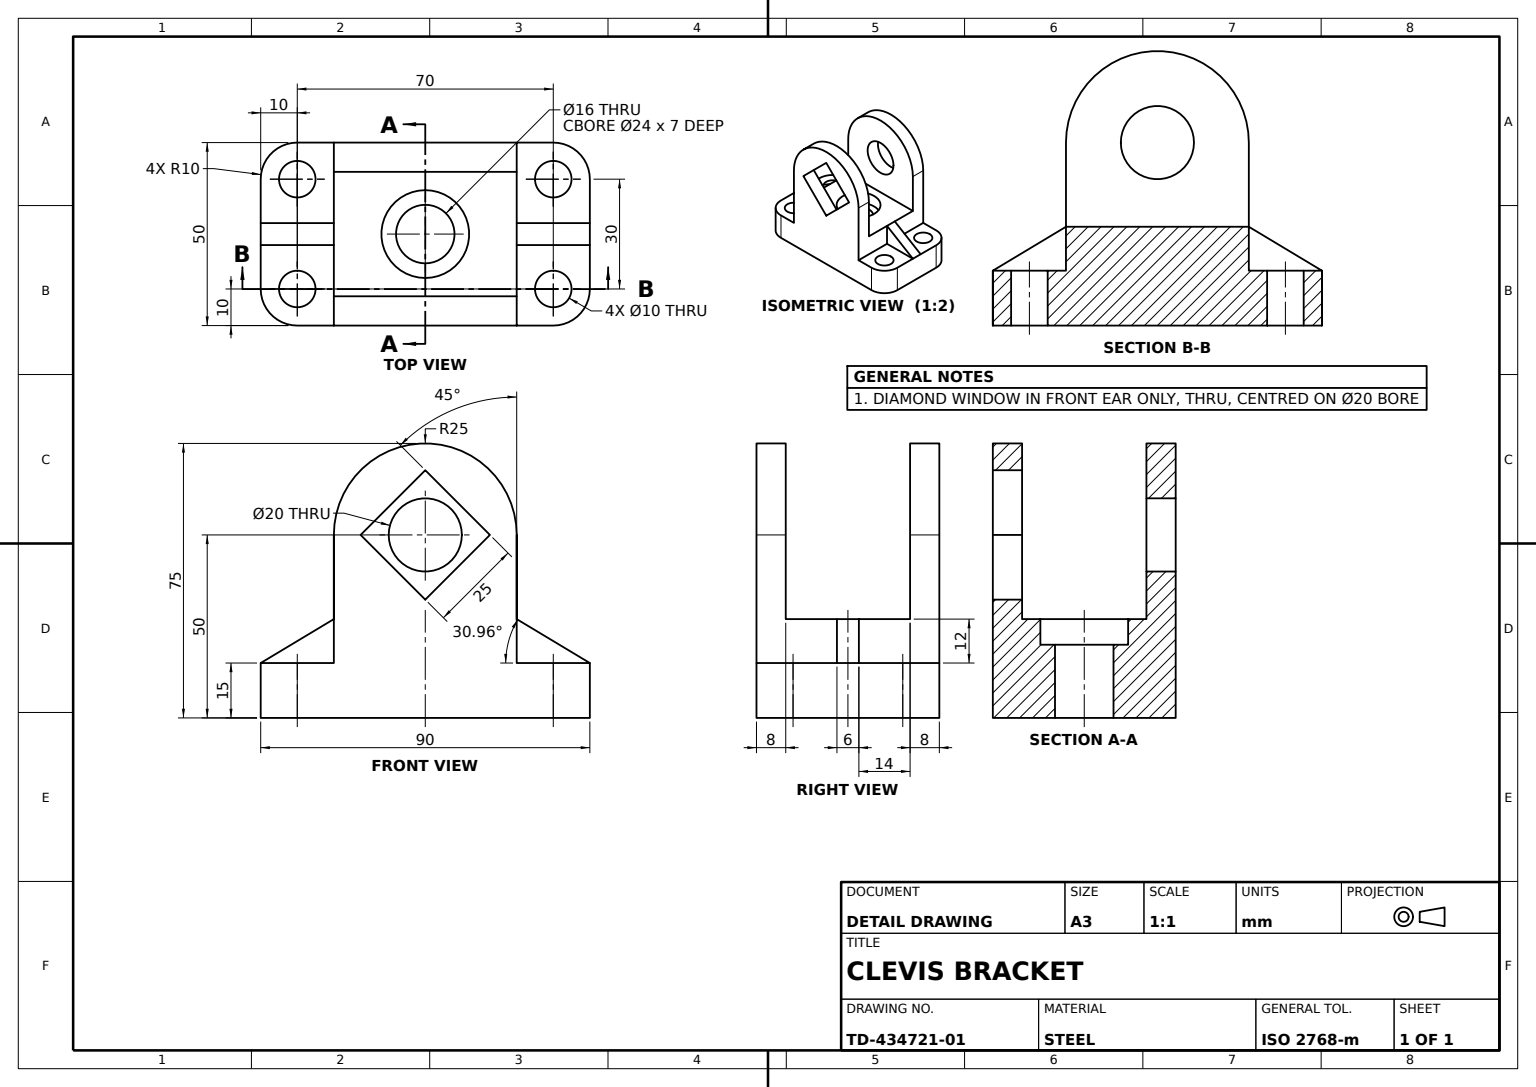
SolidWorks part; units mm, degrees
material "Plain Carbon Steel"
ref_plane "Front Plane" through (0, 0, 0) normal (0, 0, 1) x (1, 0, 0)
ref_plane "Top Plane" through (0, 0, 0) normal (0, 1, 0) x (1, 0, 0)
ref_plane "Right Plane" through (0, 0, 0) normal (1, 0, 0) x (0, 0, -1)
sketch "Base Plate Sketch" plane through (0, 0, 0) normal (0, 1, 0) x (1, 0, 0)
  line L1 (-35, -25) -> (35, -25)
  line L2 (-45, -15) -> (-45, 15)
  line L3 (-35, 25) -> (35, 25)
  line L4 (45, -15) -> (45, 15)
  line L5 (-45, -25) -> (45, 25) construction
  line L6 (-45, 25) -> (45, -25) construction
  arc A0 (-35, -25) -> (-45, -15) centre (-35, -15) cw
  arc A1 (35, -25) -> (45, -15) centre (35, -15) ccw
  arc A2 (35, 25) -> (45, 15) centre (35, 15) cw
  arc A3 (-45, 15) -> (-35, 25) centre (-35, 15) cw
  circle A4 centre (-35, 15) radius 5
  circle A5 centre (35, 15) radius 5
  circle A6 centre (-35, -15) radius 5
  circle A7 centre (35, -15) radius 5
  point P0 (0, 0)
  dimension "D2" = 10
  dimension "D4" = 10
  dimension "D1" = 50
  dimension "D3" = 70
extrude "Base Plate" add sketch "Base Plate Sketch" along normal blind 15
sketch "Clevis Ear Sketch" plane through (0, 0, 25) normal (0, 0, 1) x (1, 0, 0)
  line L0 (-25, 15) -> (-25, 50)
  line L1 (-35, 15) -> (35, 15) construction
  line L2 (25, 50) -> (25, 15)
  line L3 (-25, 15) -> (25, 15)
  arc A0 (-25, 50) -> (25, 50) centre (0, 50) cw
  dimension "D2" = 25
  dimension "D1" = 50
extrude "Clevis Ear" add sketch "Clevis Ear Sketch" against normal blind 8
mirror "Clevis Ear Mirror" about plane through (0, 0, 0) normal (0, 0, 1) of "Clevis Ear"
sketch "Centre Cut Sketch" plane through (0, 0, 25) normal (0, 0, 1) x (1, 0, 0)
  line L0 (-17.6777, 50) -> (0, 67.6777)
  line L1 (0, 67.6777) -> (17.6777, 50)
  line L2 (17.6777, 50) -> (0, 32.3223)
  line L3 (0, 32.3223) -> (-17.6777, 50)
  line L4 (0, 67.6777) -> (0, 50) construction
  line L5 (-17.6777, 50) -> (0, 50) construction
  dimension "D1" = 25
  dimension "D2" = 50
extrude "Centre Cut" cut sketch "Centre Cut Sketch" against normal blind 8
sketch "Pin Bore Sketch" plane through (0, 0, -25) normal (0, 0, -1) x (-1, 0, 0)
  circle A0 centre (0, 50) radius 10
  arc A1 (25, 50) -> (-25, 50) centre (0, 50) ccw construction
  dimension "D1" = 20
extrude "Pin Bore Ø20" cut sketch "Pin Bore Sketch" against normal blind 8
sketch "Ear Boss Sketch" plane through (0, 15, 0) normal (0, 1, 0) x (1, 0, 0)
  line L1 (-25, 17) -> (25, 17)
  line L2 (-25, 17) -> (-25, -17)
  line L3 (-25, -17) -> (25, -17)
  line L4 (25, 17) -> (25, -17)
extrude "Ear Boss" add sketch "Ear Boss Sketch" along normal blind 12
sketch "Gusset Sketch" plane through (0, 0, 0) normal (0, 0, 1) x (1, 0, 0)
  line L0 (25, 27) -> (45, 15)
rib "Gusset Rib" sketch "Gusset Sketch" sketch "Gusset Sketch" thickness 6 extrusion direction parallel to sketch draft on no parameters "D1"=6
mirror "Gusset Rib Mirror" about plane through (0, 0, 0) normal (1, 0, 0) of "Gusset Rib"
hole_wizard "Counterbored Hole Ø16" positions "3DSketch1" profile "Sketch7" legacy
sketch3d "3DSketch1"
  line L0 (-25, 27, 17) -> (25, 27, 17) construction
  line L2 (25, 27, -17) -> (-25, 27, -17) construction
  point P0 (0, 27, 0)
  point P5 (0, 27, 17)
  dimension "D1" = 17
sketch "Sketch7" plane through (0, 27, 0) normal (1, 0, 0) x (0, 0, 1)
  line L0 (0, 0) -> (0, 49.8397)
  line L1 (0, 49.8397) -> (8, 49.8397)
  line L2 (8, 49.8397) -> (8, 7)
  line L3 (8, 7) -> (12, 7)
  line L4 (12, 7) -> (12, 0)
  line L5 (12, 0) -> (0, 0)
  line L6 (0, 110) -> (0, -10) construction
  dimension "Diameter" = 16
  dimension "Depth" = 50
  dimension "C-Bore Diameter" = 24
  dimension "C-Bore Depth" = 7
